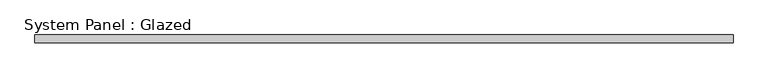
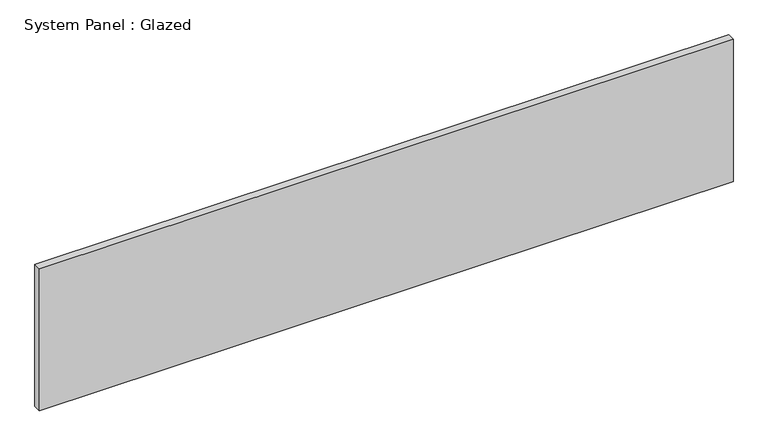
"""IFC4 building model written with IfcOpenShell, lengths in millimetres: plate geometry, System Panel : Glazed."""

from ifc_helpers import new_model, si_unit, origin, origin_with_axes, place, context, project, spatial, polyline, outline, extrude, source, transform, mapped, element, save


def system_panel_glazed_55be9c8f(model_context):
    return source(origin(), model_context, "Body", "SweptSolid", [
        extrude(outline(polyline([(1120.775, 19.05), (-1120.775, 19.05), (-1120.775, 44.45), (1120.775, 44.45), (1120.775, 19.05)])), origin_with_axes(), (0.0, 0.0, 1.0), 485.536674),
    ])


if __name__ == "__main__":
    model = new_model("IFC4")
    model_context = context("Model", 3, world=origin())
    ifc_project = project(units=[si_unit("LENGTHUNIT", "METRE", prefix="MILLI")], contexts=[model_context])
    site = spatial("IfcSite", under=ifc_project)
    building = spatial("IfcBuilding", under=site)
    placement = place(None, origin())
    system_panel_glazed_shape = system_panel_glazed_55be9c8f(model_context)
    element("IfcPlate", 1, ObjectType="System Panel : Glazed", at=placement, inside=building, context=model_context, shape_type="MappedRepresentation", body=[
        mapped(system_panel_glazed_shape, transform((0.0, 0.0, 0.0), x_axis=(1.0, 0.0, 0.0), y_axis=(0.0, 1.0, 0.0), z_axis=(0.0, 0.0, 1.0))),
    ])
    save(model, "model.ifc")

# Revit data of these elements
# Type "System Panel : Glazed"
#   Construction Type Id = "GSP4R"
#   Analytic Construction = "1/8 in Pilkington single glazing"
#   Visual Light Transmittance = 0.9
#   Solar Heat Gain Coefficient = 0.86
#   Heat Transfer Coefficient (U) = 1.18115 BTU/(h·ft²·°F)
#   Define Thermal Properties by = 1
# Element 1 (IfcPlate, "System Panel : Glazed")
#   Materials on its faces: "Glass"
# Materials
#   "Glass": class "Glass", colour RGB 0 128 192, transparency 0.75, Description = "Soda Lime Glass", Cost = 0
